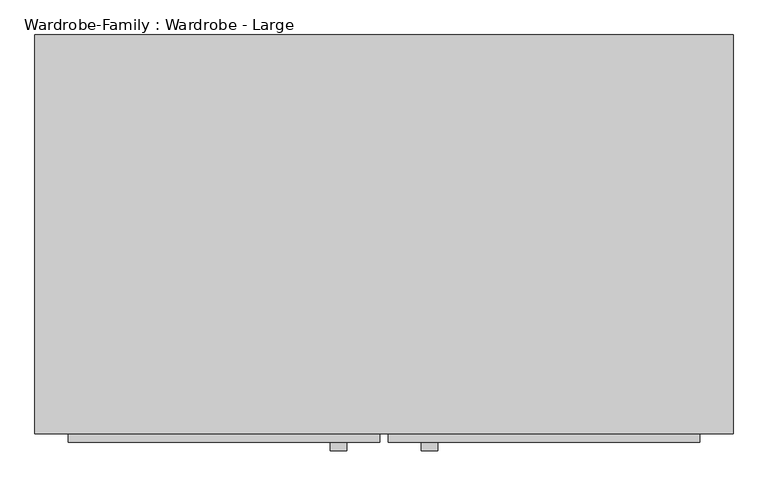
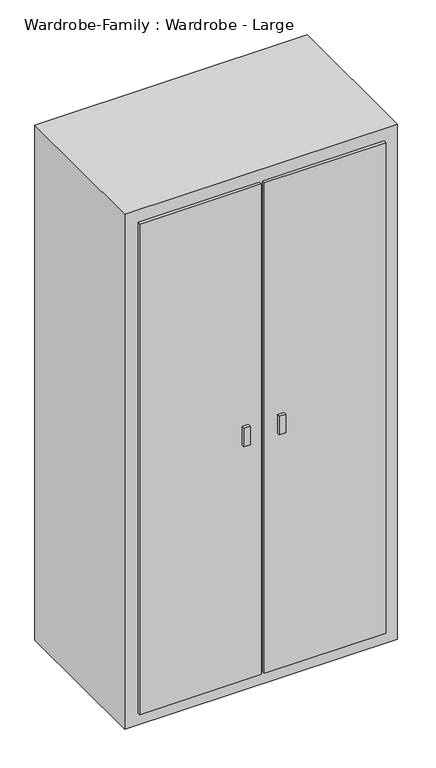
"""IFC4 building model written with IfcOpenShell, lengths in millimetres: furniture geometry, Wardrobe-Family : Wardrobe - Large."""

from ifc_helpers import new_model, si_unit, frame, origin, origin_with_axes, place, context, project, spatial, polyline, outline, extrude, source, transform, mapped, element, save


def wardrobe_family_wardrobe_large_408d0eaf(model_context):
    return source(origin(), model_context, "Body", "SweptSolid", [
        extrude(outline(polyline([(533.4, -304.8), (-533.4, -304.8), (-533.4, 304.8), (533.4, 304.8), (533.4, -304.8)])), origin_with_axes(), (0.0, 0.0, 1.0), 2133.6),
        extrude(outline(polyline([(-6.35, -304.8), (-6.35, -317.5), (-482.6, -317.5), (-482.6, -304.8), (-6.35, -304.8)])), frame((0.0, 0.0, 50.8), z_axis=(0.0, 0.0, 1.0), x_axis=(1.0, 0.0, 0.0)), (0.0, 0.0, 1.0), 2032.0),
        extrude(outline(polyline([(482.6, -317.5), (6.35, -317.5), (6.35, -304.8), (482.6, -304.8), (482.6, -317.5)])), frame((0.0, 0.0, 50.8), z_axis=(0.0, 0.0, 1.0), x_axis=(1.0, 0.0, 0.0)), (0.0, 0.0, 1.0), 2032.0),
        extrude(outline(polyline([(-57.1834134, -317.5), (-57.1834134, -330.2), (-82.3387685, -330.2), (-82.3387685, -317.5), (-57.1834134, -317.5)])), frame((0.0, 0.0, 1028.7), z_axis=(0.0, 0.0, 1.0), x_axis=(1.0, 0.0, 0.0)), (0.0, 0.0, 1.0), 76.2),
        extrude(outline(polyline([(57.1834134, -330.2), (57.1834134, -317.5), (82.3387685, -317.5), (82.3387685, -330.2), (57.1834134, -330.2)])), frame((0.0, 0.0, 1028.7), z_axis=(0.0, 0.0, 1.0), x_axis=(1.0, 0.0, 0.0)), (0.0, 0.0, 1.0), 76.2),
    ])


if __name__ == "__main__":
    model = new_model("IFC4")
    model_context = context("Model", 3, world=origin())
    ifc_project = project(units=[si_unit("LENGTHUNIT", "METRE", prefix="MILLI")], contexts=[model_context])
    site = spatial("IfcSite", under=ifc_project)
    building = spatial("IfcBuilding", under=site)
    placement = place(None, origin())
    wardrobe_family_wardrobe_large_shape = wardrobe_family_wardrobe_large_408d0eaf(model_context)
    element("IfcFurniture", 1, ObjectType="Wardrobe-Family : Wardrobe - Large", at=placement, inside=building, context=model_context, shape_type="MappedRepresentation", body=[
        mapped(wardrobe_family_wardrobe_large_shape, transform((0.0, 0.0, 0.0), x_axis=(1.0, 0.0, 0.0), y_axis=(0.0, 1.0, 0.0), z_axis=(0.0, 0.0, 1.0))),
    ])
    save(model, "model.ifc")

# Revit data of these elements
# Type "Wardrobe-Family : Wardrobe - Large"
#   Width = 2.0 ft
#   Length = 3.5 ft
#   Default Elevation = 0
# Element 1 (IfcFurniture, "Wardrobe-Family : Wardrobe - Large")
#   Materials on its faces: "Wood Material", "Steel Handle"
# Materials
#   "Wood Material": class "Generic", colour RGB 128 72 40, transparency 0, Cost = 0
#   "Steel Handle": class "Generic", colour RGB 206 211 212, transparency 0, Cost = 0
